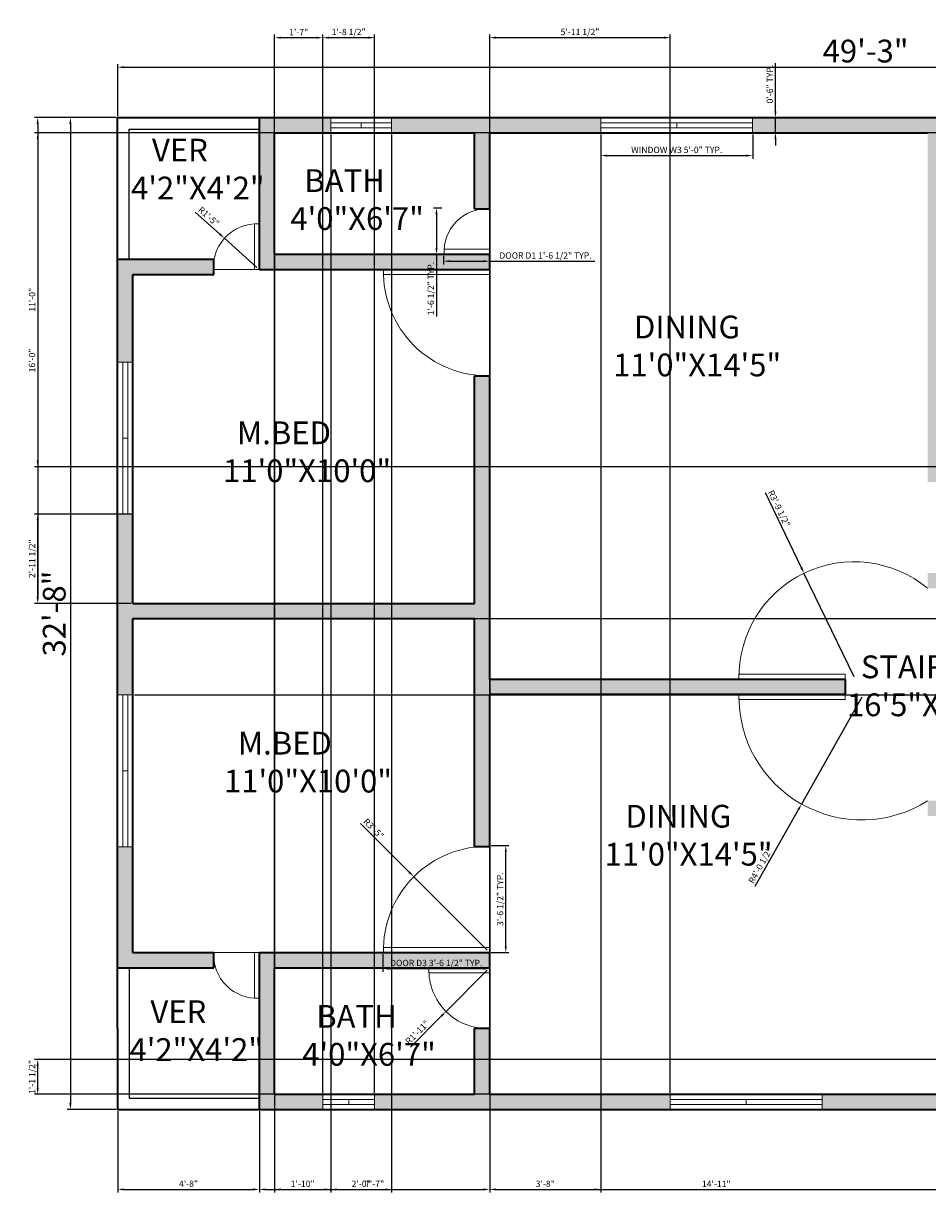
# Model space of a CAD drawing. Units: inches. Extents: x 5145 to 5807, y 9597 to 10060.
# Tile 1 of 3: x 5145 to 5502, y 9597 to 10060. Entities that reach past the tile are written whole.
import ezdxf

# ---------------------------------------------------------------- set-up
doc = ezdxf.new("R2010")
doc.units = ezdxf.units.IN
for name, color, linetype, lineweight in [('A-ANNO-DIMS', 7, 'Continuous', 18), ('A-AREA-IDEN', 7, 'Continuous', 18), ('A-GLAZ', 140, 'Continuous', 18), ('A-WALL', 7, 'Continuous', 35)]:
    doc.layers.add(name, color=color, linetype=linetype, lineweight=lineweight)
for name, color, linetype, lineweight, true_color in [('A-DOOR', 2, 'Continuous', 18, 0xf1eb1f), ('A-WALL-PATT', 159, 'Continuous', 13, 0x22346e), ('A-WALL-PRPT', 61, 'Continuous', 25, 0xedee99)]:
    doc.layers.add(name, color=color, linetype=linetype, lineweight=lineweight, true_color=true_color)
doc.styles.get("Standard").update_dxf_attribs({"font": 'arial.ttf'})
doc.dimstyles.new('ISO-25', dxfattribs={"dimtxt": 2.5, "dimasz": 2.5, "dimexe": 1.25, "dimexo": 0.625, "dimtad": 1, "dimlunit": 3, "dimtxsty": 'Standard', "dimcen": 2.5, "dimadec": 0, "dimazin": 0, "dimtfac": 1, "dimtmove": 0, "dimatfit": 3, "dimfxl": 1, "dimarcsym": 0})

# ---------------------------------------------------------------- blocks, each defined once
blk = doc.blocks.new('*D1')
at = {"layer": 'A-ANNO-DIMS', "color": 0, "lineweight": -2, "transparency": 16777216}
for p, q in [((5182.12, 10022.89), (5182.12, 10043.44)), ((5184.62, 10042.19), (5770.62, 10042.19)), ((5773.12, 10022.89), (5773.12, 10043.44))]:
    blk.add_line(p, q, dxfattribs=at)
at = {"layer": 'A-ANNO-DIMS', "color": 0, "transparency": 16777216}
for points in [[(5184.62, 10042.6), (5184.62, 10041.77), (5182.12, 10042.19)], [(5770.62, 10042.6), (5770.62, 10041.77), (5773.12, 10042.19)]]:
    blk.add_solid(points, dxfattribs=at)
at = {"layer": 'Defpoints', "color": 0, "transparency": 16777216}
for p in [(5773.12, 10042.19), (5182.12, 10022.27), (5773.12, 10022.27)]:
    blk.add_point(p, dxfattribs=at)
at = {"layer": 'A-ANNO-DIMS', "color": 0, "transparency": 16777216, "insert": (5477.62, 10047.41), "char_height": 9, "attachment_point": 5}
blk.add_mtext('49\'-3"', dxfattribs=at)
blk = doc.blocks.new('*D2')
at = {"layer": 'A-ANNO-DIMS', "color": 0, "lineweight": -2, "transparency": 16777216}
for p, q in [((5181.49, 10022.27), (5162.2, 10022.27)), ((5163.45, 10019.77), (5163.45, 9632.77)), ((5181.49, 9630.27), (5162.2, 9630.27))]:
    blk.add_line(p, q, dxfattribs=at)
at = {"layer": 'A-ANNO-DIMS', "color": 0, "transparency": 16777216}
for points in [[(5163.03, 10019.77), (5163.86, 10019.77), (5163.45, 10022.27)], [(5163.03, 9632.77), (5163.86, 9632.77), (5163.45, 9630.27)]]:
    blk.add_solid(points, dxfattribs=at)
at = {"layer": 'Defpoints', "color": 0, "transparency": 16777216}
for p in [(5182.12, 10022.27), (5163.45, 9630.27), (5182.12, 9630.27)]:
    blk.add_point(p, dxfattribs=at)
at = {"layer": 'A-ANNO-DIMS', "color": 0, "transparency": 16777216, "insert": (5158.22, 9826.27), "char_height": 9, "attachment_point": 5, "rotation": 90}
blk.add_mtext('32\'-8"', dxfattribs=at)
blk = doc.blocks.new('WIN-60IN')
for p, q in [((0, 6), (0, 0)), ((0, 6), (60, 6)), ((60, 0), (60, 6)), ((0, 4), (60, 4)), ((0, 2), (60, 2)), ((60, 0), (0, 0)), ((30, 2), (30, 4))]:
    blk.add_line(p, q)
blk = doc.blocks.new('DOOR-SWING-18IN')
for p, q in [((0.03, 18.03), (18.03, 18.03)), ((16.03, 0.03), (16.03, 18.03)), ((16.03, 18.03), (18.03, 18.03)), ((18.03, 18.03), (18.03, 0.03)), ((18.03, 0.03), (16.03, 0.03))]:
    blk.add_line(p, q)
blk.add_arc((17.03, 17.03), 17.03, 176.6335, 273.3665)
blk = doc.blocks.new('DOOR-SWING-42IN')
for p, q in [((42.01, 0), (42.01, 42)), ((0.01, 0), (0.01, 2)), ((0.01, 2), (42.01, 2)), ((42.01, 0), (0.01, 0)), ((42.01, 2), (42.01, 0))]:
    blk.add_line(p, q)
blk.add_arc((41.01, 1), 41.01, 88.6028, 181.3972)
blk = doc.blocks.new('*D13')
at = {"layer": 'A-ANNO-DIMS', "color": 0, "lineweight": -2, "transparency": 16777216}
for p, q in [((5373, 10015.64), (5373, 10006.02)), ((5433, 10015.64), (5433, 10006.02)), ((5375.5, 10007.27), (5430.5, 10007.27))]:
    blk.add_line(p, q, dxfattribs=at)
at = {"layer": 'A-ANNO-DIMS', "color": 0, "transparency": 16777216}
for points in [[(5375.5, 10007.68), (5375.5, 10006.85), (5373, 10007.27)], [(5430.5, 10007.68), (5430.5, 10006.85), (5433, 10007.27)]]:
    blk.add_solid(points, dxfattribs=at)
at = {"layer": 'Defpoints', "color": 0, "transparency": 16777216}
for p in [(5373, 10016.27), (5433, 10016.27), (5433, 10007.27)]:
    blk.add_point(p, dxfattribs=at)
at = {"layer": 'A-ANNO-DIMS', "color": 0, "transparency": 16777216, "insert": (5403, 10009.19), "char_height": 2.5, "attachment_point": 5}
blk.add_mtext('WINDOW W3 5\'-0" TYP.', dxfattribs=at)
blk = doc.blocks.new('*D14')
at = {"layer": 'A-ANNO-DIMS', "color": 0, "lineweight": -2, "transparency": 16777216}
for p, q in [((5442, 10024.77), (5442, 10043.76)), ((5433.62, 10022.27), (5443.25, 10022.27)), ((5442, 10016.27), (5442, 10022.27)), ((5433.62, 10016.27), (5443.25, 10016.27)), ((5442, 10013.77), (5442, 10011.27))]:
    blk.add_line(p, q, dxfattribs=at)
at = {"layer": 'A-ANNO-DIMS', "color": 0, "transparency": 16777216}
for points in [[(5441.58, 10024.77), (5442.41, 10024.77), (5442, 10022.27)], [(5441.58, 10013.77), (5442.41, 10013.77), (5442, 10016.27)]]:
    blk.add_solid(points, dxfattribs=at)
at = {"layer": 'Defpoints', "color": 0, "transparency": 16777216}
for p in [(5433, 10022.27), (5442, 10022.27), (5433, 10016.27)]:
    blk.add_point(p, dxfattribs=at)
at = {"layer": 'A-ANNO-DIMS', "color": 0, "transparency": 16777216, "insert": (5440.09, 10035.51), "char_height": 2.5, "attachment_point": 5, "rotation": 90}
blk.add_mtext('0\'-6" TYP.', dxfattribs=at)
blk = doc.blocks.new('*D15')
at = {"layer": 'A-ANNO-DIMS', "color": 0, "lineweight": -2, "transparency": 16777216}
for p, q in [((5310.83, 9967.64), (5310.83, 9964.27)), ((5329.12, 9967.64), (5329.12, 9964.27)), ((5313.33, 9965.52), (5326.62, 9965.52)), ((5329.12, 9965.52), (5370.69, 9965.52))]:
    blk.add_line(p, q, dxfattribs=at)
at = {"layer": 'A-ANNO-DIMS', "color": 0, "transparency": 16777216}
for points in [[(5313.33, 9965.94), (5313.33, 9965.11), (5310.83, 9965.52)], [(5326.62, 9965.94), (5326.62, 9965.11), (5329.12, 9965.52)]]:
    blk.add_solid(points, dxfattribs=at)
at = {"layer": 'Defpoints', "color": 0, "transparency": 16777216}
for p in [(5310.83, 9968.27), (5329.12, 9968.27), (5329.12, 9965.52)]:
    blk.add_point(p, dxfattribs=at)
at = {"layer": 'A-ANNO-DIMS', "color": 0, "transparency": 16777216, "insert": (5351.15, 9967.44), "char_height": 2.5, "attachment_point": 5}
blk.add_mtext('DOOR D1 1\'-6 1/2" TYP.', dxfattribs=at)
blk = doc.blocks.new('*D16')
at = {"layer": 'A-ANNO-DIMS', "color": 0, "lineweight": -2, "transparency": 16777216}
for p, q in [((5310.21, 9986.55), (5306.84, 9986.55)), ((5308.09, 9984.05), (5308.09, 9970.77)), ((5310.21, 9968.27), (5306.84, 9968.27)), ((5308.09, 9968.27), (5308.09, 9943.69))]:
    blk.add_line(p, q, dxfattribs=at)
at = {"layer": 'A-ANNO-DIMS', "color": 0, "transparency": 16777216}
for points in [[(5307.67, 9984.05), (5308.5, 9984.05), (5308.09, 9986.55)], [(5307.67, 9970.77), (5308.5, 9970.77), (5308.09, 9968.27)]]:
    blk.add_solid(points, dxfattribs=at)
at = {"layer": 'Defpoints', "color": 0, "transparency": 16777216}
for p in [(5310.83, 9986.55), (5308.09, 9968.27), (5310.83, 9968.27)]:
    blk.add_point(p, dxfattribs=at)
at = {"layer": 'A-ANNO-DIMS', "color": 0, "transparency": 16777216, "insert": (5306.17, 9954.73), "char_height": 2.5, "attachment_point": 5, "rotation": 90}
blk.add_mtext('1\'-6 1/2" TYP.', dxfattribs=at)
blk = doc.blocks.new('*D19')
at = {"layer": 'A-ANNO-DIMS', "color": 0, "lineweight": -2, "transparency": 16777216}
for p, q in [((5286.84, 9691.64), (5286.84, 9684.68)), ((5329.12, 9691.64), (5329.12, 9684.68)), ((5289.34, 9685.93), (5326.62, 9685.93))]:
    blk.add_line(p, q, dxfattribs=at)
at = {"layer": 'A-ANNO-DIMS', "color": 0, "transparency": 16777216}
for points in [[(5289.34, 9686.34), (5289.34, 9685.51), (5286.84, 9685.93)], [(5326.62, 9686.34), (5326.62, 9685.51), (5329.12, 9685.93)]]:
    blk.add_solid(points, dxfattribs=at)
at = {"layer": 'Defpoints', "color": 0, "transparency": 16777216}
for p in [(5286.84, 9692.27), (5329.12, 9692.27), (5329.12, 9685.93)]:
    blk.add_point(p, dxfattribs=at)
at = {"layer": 'A-ANNO-DIMS', "color": 0, "transparency": 16777216, "insert": (5307.98, 9687.85), "char_height": 2.5, "attachment_point": 5}
blk.add_mtext('DOOR D3 3\'-6 1/2" TYP.', dxfattribs=at)
blk = doc.blocks.new('*D20')
at = {"layer": 'A-ANNO-DIMS', "color": 0, "lineweight": -2, "transparency": 16777216}
for p, q in [((5329.74, 9734.54), (5336.71, 9734.54)), ((5335.46, 9694.77), (5335.46, 9732.04)), ((5329.74, 9692.27), (5336.71, 9692.27))]:
    blk.add_line(p, q, dxfattribs=at)
at = {"layer": 'A-ANNO-DIMS', "color": 0, "transparency": 16777216}
for points in [[(5335.04, 9732.04), (5335.87, 9732.04), (5335.46, 9734.54)], [(5335.04, 9694.77), (5335.87, 9694.77), (5335.46, 9692.27)]]:
    blk.add_solid(points, dxfattribs=at)
at = {"layer": 'Defpoints', "color": 0, "transparency": 16777216}
for p in [(5329.12, 9734.54), (5335.46, 9734.54), (5329.12, 9692.27)]:
    blk.add_point(p, dxfattribs=at)
at = {"layer": 'A-ANNO-DIMS', "color": 0, "transparency": 16777216, "insert": (5333.54, 9713.4), "char_height": 2.5, "attachment_point": 5, "rotation": 90}
blk.add_mtext('3\'-6 1/2" TYP.', dxfattribs=at)
blk = doc.blocks.new('*D21')
at = {"layer": 'A-ANNO-DIMS', "color": 0, "lineweight": -2, "transparency": 16777216}
for p, q in [((5182.12, 9629.64), (5182.12, 9597.42)), ((5238.12, 9629.64), (5238.12, 9597.42)), ((5184.62, 9598.67), (5235.62, 9598.67))]:
    blk.add_line(p, q, dxfattribs=at)
at = {"layer": 'A-ANNO-DIMS', "color": 0, "transparency": 16777216}
for points in [[(5184.62, 9599.08), (5184.62, 9598.25), (5182.12, 9598.67)], [(5235.62, 9599.08), (5235.62, 9598.25), (5238.12, 9598.67)]]:
    blk.add_solid(points, dxfattribs=at)
at = {"layer": 'Defpoints', "color": 0, "transparency": 16777216}
for p in [(5182.12, 9630.27), (5238.12, 9630.27), (5238.12, 9598.67)]:
    blk.add_point(p, dxfattribs=at)
at = {"layer": 'A-ANNO-DIMS', "color": 0, "transparency": 16777216, "insert": (5210.12, 9600.57), "char_height": 2.5, "attachment_point": 5}
blk.add_mtext('4\'-8"', dxfattribs=at)
blk = doc.blocks.new('*D22')
at = {"layer": 'A-ANNO-DIMS', "color": 0, "lineweight": -2, "transparency": 16777216}
for p, q in [((5329.12, 9635.64), (5329.12, 9597.42)), ((5238.12, 9629.64), (5238.12, 9597.42)), ((5240.62, 9598.67), (5326.62, 9598.67))]:
    blk.add_line(p, q, dxfattribs=at)
at = {"layer": 'A-ANNO-DIMS', "color": 0, "transparency": 16777216}
for points in [[(5240.62, 9599.08), (5240.62, 9598.25), (5238.12, 9598.67)], [(5326.62, 9599.08), (5326.62, 9598.25), (5329.12, 9598.67)]]:
    blk.add_solid(points, dxfattribs=at)
at = {"layer": 'Defpoints', "color": 0, "transparency": 16777216}
for p in [(5329.12, 9636.27), (5238.12, 9630.27), (5329.12, 9598.67)]:
    blk.add_point(p, dxfattribs=at)
at = {"layer": 'A-ANNO-DIMS', "color": 0, "transparency": 16777216, "insert": (5283.62, 9600.54), "char_height": 2.5, "attachment_point": 5}
blk.add_mtext('7\'-7"', dxfattribs=at)
blk = doc.blocks.new('*D23')
at = {"layer": 'A-ANNO-DIMS', "color": 0, "lineweight": -2, "transparency": 16777216}
for p, q in [((5329.12, 9635.64), (5329.12, 9597.42)), ((5508.12, 9635.64), (5508.12, 9597.42)), ((5331.62, 9598.67), (5505.62, 9598.67))]:
    blk.add_line(p, q, dxfattribs=at)
at = {"layer": 'A-ANNO-DIMS', "color": 0, "transparency": 16777216}
for points in [[(5331.62, 9599.08), (5331.62, 9598.25), (5329.12, 9598.67)], [(5505.62, 9599.08), (5505.62, 9598.25), (5508.12, 9598.67)]]:
    blk.add_solid(points, dxfattribs=at)
at = {"layer": 'Defpoints', "color": 0, "transparency": 16777216}
for p in [(5329.12, 9636.27), (5508.12, 9636.27), (5508.12, 9598.67)]:
    blk.add_point(p, dxfattribs=at)
at = {"layer": 'A-ANNO-DIMS', "color": 0, "transparency": 16777216, "insert": (5418.62, 9600.55), "char_height": 2.5, "attachment_point": 5}
blk.add_mtext('14\'-11"', dxfattribs=at)
blk = doc.blocks.new('*D29')
at = {"layer": 'A-ANNO-DIMS', "color": 0, "lineweight": -2, "transparency": 16777216}
for p, q in [((5590.49, 10016.27), (5149.27, 10016.27)), ((5150.52, 10013.77), (5150.52, 9886.77)), ((5590.49, 9884.27), (5149.27, 9884.27))]:
    blk.add_line(p, q, dxfattribs=at)
at = {"layer": 'A-ANNO-DIMS', "color": 0, "transparency": 16777216}
for points in [[(5150.1, 10013.77), (5150.93, 10013.77), (5150.52, 10016.27)], [(5150.1, 9886.77), (5150.93, 9886.77), (5150.52, 9884.27)]]:
    blk.add_solid(points, dxfattribs=at)
at = {"layer": 'Defpoints', "color": 0, "transparency": 16777216}
for p in [(5591.12, 10016.27), (5150.52, 9884.27), (5591.12, 9884.27)]:
    blk.add_point(p, dxfattribs=at)
at = {"layer": 'A-ANNO-DIMS', "color": 0, "transparency": 16777216, "insert": (5148.61, 9950.27), "char_height": 2.5, "attachment_point": 5, "rotation": 90}
blk.add_mtext('11\'-0"', dxfattribs=at)
blk = doc.blocks.new('*D33')
at = {"layer": 'A-ANNO-DIMS', "color": 0, "lineweight": -2, "transparency": 16777216}
for p, q in [((5181.49, 10022.27), (5149.27, 10022.27)), ((5150.52, 10019.77), (5150.52, 9832.77)), ((5187.49, 9830.27), (5149.27, 9830.27))]:
    blk.add_line(p, q, dxfattribs=at)
at = {"layer": 'A-ANNO-DIMS', "color": 0, "transparency": 16777216}
for points in [[(5150.1, 10019.77), (5150.93, 10019.77), (5150.52, 10022.27)], [(5150.1, 9832.77), (5150.93, 9832.77), (5150.52, 9830.27)]]:
    blk.add_solid(points, dxfattribs=at)
at = {"layer": 'Defpoints', "color": 0, "transparency": 16777216}
for p in [(5182.12, 10022.27), (5150.52, 9830.27), (5188.12, 9830.27)]:
    blk.add_point(p, dxfattribs=at)
at = {"layer": 'A-ANNO-DIMS', "color": 0, "transparency": 16777216, "insert": (5148.61, 9926.27), "char_height": 2.5, "attachment_point": 5, "rotation": 90}
blk.add_mtext('16\'-0"', dxfattribs=at)
blk = doc.blocks.new('*D34')
at = {"layer": 'A-ANNO-DIMS', "color": 0, "lineweight": -2, "transparency": 16777216}
for p, q in [((5244.12, 10015.64), (5244.12, 9597.42)), ((5266.31, 10015.64), (5266.31, 9597.42)), ((5246.62, 9598.67), (5263.81, 9598.67))]:
    blk.add_line(p, q, dxfattribs=at)
at = {"layer": 'A-ANNO-DIMS', "color": 0, "transparency": 16777216}
for points in [[(5246.62, 9599.08), (5246.62, 9598.25), (5244.12, 9598.67)], [(5263.81, 9599.08), (5263.81, 9598.25), (5266.31, 9598.67)]]:
    blk.add_solid(points, dxfattribs=at)
at = {"layer": 'Defpoints', "color": 0, "transparency": 16777216}
for p in [(5244.12, 10016.27), (5266.31, 10016.27), (5266.31, 9598.67)]:
    blk.add_point(p, dxfattribs=at)
at = {"layer": 'A-ANNO-DIMS', "color": 0, "transparency": 16777216, "insert": (5255.21, 9600.57), "char_height": 2.5, "attachment_point": 5}
blk.add_mtext('1\'-10"', dxfattribs=at)
blk = doc.blocks.new('*D35')
at = {"layer": 'A-ANNO-DIMS', "color": 0, "lineweight": -2, "transparency": 16777216}
for p, q in [((5266.31, 10015.64), (5266.31, 9597.42)), ((5290.31, 10015.64), (5290.31, 9597.42)), ((5268.81, 9598.67), (5287.81, 9598.67))]:
    blk.add_line(p, q, dxfattribs=at)
at = {"layer": 'A-ANNO-DIMS', "color": 0, "transparency": 16777216}
for points in [[(5268.81, 9599.08), (5268.81, 9598.25), (5266.31, 9598.67)], [(5287.81, 9599.08), (5287.81, 9598.25), (5290.31, 9598.67)]]:
    blk.add_solid(points, dxfattribs=at)
at = {"layer": 'Defpoints', "color": 0, "transparency": 16777216}
for p in [(5266.31, 10016.27), (5290.31, 10016.27), (5290.31, 9598.67)]:
    blk.add_point(p, dxfattribs=at)
at = {"layer": 'A-ANNO-DIMS', "color": 0, "transparency": 16777216, "insert": (5278.31, 9600.57), "char_height": 2.5, "attachment_point": 5}
blk.add_mtext('2\'-0"', dxfattribs=at)
blk = doc.blocks.new('*D36')
at = {"layer": 'A-ANNO-DIMS', "color": 0, "lineweight": -2, "transparency": 16777216}
for p, q in [((5329.12, 10015.64), (5329.12, 9597.42)), ((5373, 10015.64), (5373, 9597.42)), ((5331.62, 9598.67), (5370.5, 9598.67))]:
    blk.add_line(p, q, dxfattribs=at)
at = {"layer": 'A-ANNO-DIMS', "color": 0, "transparency": 16777216}
for points in [[(5331.62, 9599.08), (5331.62, 9598.25), (5329.12, 9598.67)], [(5370.5, 9599.08), (5370.5, 9598.25), (5373, 9598.67)]]:
    blk.add_solid(points, dxfattribs=at)
at = {"layer": 'Defpoints', "color": 0, "transparency": 16777216}
for p in [(5329.12, 10016.27), (5373, 10016.27), (5373, 9598.67)]:
    blk.add_point(p, dxfattribs=at)
at = {"layer": 'A-ANNO-DIMS', "color": 0, "transparency": 16777216, "insert": (5351.06, 9600.57), "char_height": 2.5, "attachment_point": 5}
blk.add_mtext('3\'-8"', dxfattribs=at)
blk = doc.blocks.new('*D40')
at = {"layer": 'A-ANNO-DIMS', "color": 0, "lineweight": -2, "transparency": 16777216}
for p, q in [((5244.12, 9636.89), (5244.12, 10055.12)), ((5246.62, 10053.87), (5260.67, 10053.87)), ((5263.17, 9636.89), (5263.17, 10055.12))]:
    blk.add_line(p, q, dxfattribs=at)
at = {"layer": 'A-ANNO-DIMS', "color": 0, "transparency": 16777216}
for points in [[(5246.62, 10054.28), (5246.62, 10053.45), (5244.12, 10053.87)], [(5260.67, 10054.28), (5260.67, 10053.45), (5263.17, 10053.87)]]:
    blk.add_solid(points, dxfattribs=at)
at = {"layer": 'Defpoints', "color": 0, "transparency": 16777216}
for p in [(5263.17, 10053.87), (5244.12, 9636.27), (5263.17, 9636.27)]:
    blk.add_point(p, dxfattribs=at)
at = {"layer": 'A-ANNO-DIMS', "color": 0, "transparency": 16777216, "insert": (5253.64, 10055.75), "char_height": 2.5, "attachment_point": 5}
blk.add_mtext('1\'-7"', dxfattribs=at)
blk = doc.blocks.new('*D41')
at = {"layer": 'A-ANNO-DIMS', "color": 0, "lineweight": -2, "transparency": 16777216}
for p, q in [((5263.17, 9636.89), (5263.17, 10055.12)), ((5265.67, 10053.87), (5281.12, 10053.87)), ((5283.62, 9636.89), (5283.62, 10055.12))]:
    blk.add_line(p, q, dxfattribs=at)
at = {"layer": 'A-ANNO-DIMS', "color": 0, "transparency": 16777216}
for points in [[(5265.67, 10054.28), (5265.67, 10053.45), (5263.17, 10053.87)], [(5281.12, 10054.28), (5281.12, 10053.45), (5283.62, 10053.87)]]:
    blk.add_solid(points, dxfattribs=at)
at = {"layer": 'Defpoints', "color": 0, "transparency": 16777216}
for p in [(5283.62, 10053.87), (5263.17, 9636.27), (5283.62, 9636.27)]:
    blk.add_point(p, dxfattribs=at)
at = {"layer": 'A-ANNO-DIMS', "color": 0, "transparency": 16777216, "insert": (5273.39, 10055.79), "char_height": 2.5, "attachment_point": 5}
blk.add_mtext('1\'-8 1/2"', dxfattribs=at)
blk = doc.blocks.new('*D42')
at = {"layer": 'A-ANNO-DIMS', "color": 0, "lineweight": -2, "transparency": 16777216}
for p, q in [((5329.12, 9636.89), (5329.12, 10055.12)), ((5331.62, 10053.87), (5397.94, 10053.87)), ((5400.44, 9636.89), (5400.44, 10055.12))]:
    blk.add_line(p, q, dxfattribs=at)
at = {"layer": 'A-ANNO-DIMS', "color": 0, "transparency": 16777216}
for points in [[(5331.62, 10054.28), (5331.62, 10053.45), (5329.12, 10053.87)], [(5397.94, 10054.28), (5397.94, 10053.45), (5400.44, 10053.87)]]:
    blk.add_solid(points, dxfattribs=at)
at = {"layer": 'Defpoints', "color": 0, "transparency": 16777216}
for p in [(5400.44, 10053.87), (5329.12, 9636.27), (5400.44, 9636.27)]:
    blk.add_point(p, dxfattribs=at)
at = {"layer": 'A-ANNO-DIMS', "color": 0, "transparency": 16777216, "insert": (5364.78, 10055.79), "char_height": 2.5, "attachment_point": 5}
blk.add_mtext('5\'-11 1/2"', dxfattribs=at)
blk = doc.blocks.new('*D45')
at = {"layer": 'A-ANNO-DIMS', "color": 0, "lineweight": -2, "transparency": 16777216}
for p, q in [((5187.49, 9865.61), (5149.27, 9865.61)), ((5150.52, 9832.77), (5150.52, 9863.11)), ((5187.49, 9830.27), (5149.27, 9830.27))]:
    blk.add_line(p, q, dxfattribs=at)
at = {"layer": 'A-ANNO-DIMS', "color": 0, "transparency": 16777216}
for points in [[(5150.1, 9863.11), (5150.93, 9863.11), (5150.52, 9865.61)], [(5150.1, 9832.77), (5150.93, 9832.77), (5150.52, 9830.27)]]:
    blk.add_solid(points, dxfattribs=at)
at = {"layer": 'Defpoints', "color": 0, "transparency": 16777216}
for p in [(5150.52, 9865.61), (5188.12, 9865.61), (5188.12, 9830.27)]:
    blk.add_point(p, dxfattribs=at)
at = {"layer": 'A-ANNO-DIMS', "color": 0, "transparency": 16777216, "insert": (5148.6, 9847.94), "char_height": 2.5, "attachment_point": 5, "rotation": 90}
blk.add_mtext('2\'-11 1/2"', dxfattribs=at)
blk = doc.blocks.new('*D46')
at = {"layer": 'A-ANNO-DIMS', "color": 0, "lineweight": -2, "transparency": 16777216}
for p, q in [((5188.74, 9824.27), (5805.97, 9824.27)), ((5804.72, 9821.77), (5804.72, 9796.64)), ((5188.74, 9794.14), (5805.97, 9794.14))]:
    blk.add_line(p, q, dxfattribs=at)
at = {"layer": 'A-ANNO-DIMS', "color": 0, "transparency": 16777216}
for points in [[(5804.3, 9821.77), (5805.13, 9821.77), (5804.72, 9824.27)], [(5804.3, 9796.64), (5805.13, 9796.64), (5804.72, 9794.14)]]:
    blk.add_solid(points, dxfattribs=at)
at = {"layer": 'Defpoints', "color": 0, "transparency": 16777216}
for p in [(5188.12, 9824.27), (5188.12, 9794.14), (5804.72, 9794.14)]:
    blk.add_point(p, dxfattribs=at)
at = {"layer": 'A-ANNO-DIMS', "color": 0, "transparency": 16777216, "insert": (5802.81, 9809.2), "char_height": 2.5, "attachment_point": 5, "rotation": 90}
blk.add_mtext('2\'-6"', dxfattribs=at)
blk = doc.blocks.new('*D49')
at = {"layer": 'A-ANNO-DIMS', "color": 0, "lineweight": -2, "transparency": 16777216}
for p, q in [((5724.49, 9649.99), (5149.27, 9649.99)), ((5150.52, 9638.77), (5150.52, 9647.49)), ((5724.49, 9636.27), (5149.27, 9636.27))]:
    blk.add_line(p, q, dxfattribs=at)
at = {"layer": 'A-ANNO-DIMS', "color": 0, "transparency": 16777216}
for points in [[(5150.1, 9647.49), (5150.93, 9647.49), (5150.52, 9649.99)], [(5150.1, 9638.77), (5150.93, 9638.77), (5150.52, 9636.27)]]:
    blk.add_solid(points, dxfattribs=at)
at = {"layer": 'Defpoints', "color": 0, "transparency": 16777216}
for p in [(5150.52, 9649.99), (5725.12, 9649.99), (5725.12, 9636.27)]:
    blk.add_point(p, dxfattribs=at)
at = {"layer": 'A-ANNO-DIMS', "color": 0, "transparency": 16777216, "insert": (5148.6, 9643.13), "char_height": 2.5, "attachment_point": 5, "rotation": 90}
blk.add_mtext('1\'-1 1/2"', dxfattribs=at)
blk = doc.blocks.new('*D50')
at = {"layer": 'A-ANNO-DIMS', "color": 0, "lineweight": -2, "transparency": 16777216}
for p, q in [((5476.13, 9793.27), (5452.29, 9750.98)), ((5434.04, 9718.58), (5451.06, 9748.8))]:
    blk.add_line(p, q, dxfattribs=at)
at = {"layer": 'A-ANNO-DIMS', "color": 0, "transparency": 16777216}
blk.add_solid([(5450.7, 9749), (5451.43, 9748.59), (5452.29, 9750.98)], dxfattribs=at)
at = {"layer": 'Defpoints', "color": 0, "transparency": 16777216}
for p in [(5476.13, 9793.27), (5452.29, 9750.98)]:
    blk.add_point(p, dxfattribs=at)
at = {"layer": 'A-ANNO-DIMS', "color": 0, "transparency": 16777216, "insert": (5436.32, 9726.55), "char_height": 2.5, "attachment_point": 5, "rotation": 60.5951}
blk.add_mtext('R4\'-0 1/2"', dxfattribs=at)
blk = doc.blocks.new('*D51')
at = {"layer": 'A-ANNO-DIMS', "color": 0, "lineweight": -2, "transparency": 16777216}
for p, q in [((5437.91, 9874.05), (5452.19, 9844.48)), ((5473.07, 9801.27), (5453.28, 9842.22))]:
    blk.add_line(p, q, dxfattribs=at)
at = {"layer": 'A-ANNO-DIMS', "color": 0, "transparency": 16777216}
blk.add_solid([(5452.57, 9844.66), (5451.82, 9844.29), (5453.28, 9842.22)], dxfattribs=at)
at = {"layer": 'Defpoints', "color": 0, "transparency": 16777216}
for p in [(5453.28, 9842.22), (5473.07, 9801.27)]:
    blk.add_point(p, dxfattribs=at)
at = {"layer": 'A-ANNO-DIMS', "color": 0, "transparency": 16777216, "insert": (5443.14, 9867.63), "char_height": 2.5, "attachment_point": 5, "rotation": 295.7836}
blk.add_mtext('R3\'-9 1/2"', dxfattribs=at)
blk = doc.blocks.new('*D52')
at = {"layer": 'A-ANNO-DIMS', "color": 0, "lineweight": -2, "transparency": 16777216}
for p, q in [((5278.08, 9743.3), (5297.35, 9724.03)), ((5328.12, 9693.27), (5299.12, 9722.27))]:
    blk.add_line(p, q, dxfattribs=at)
at = {"layer": 'A-ANNO-DIMS', "color": 0, "transparency": 16777216}
blk.add_solid([(5297.64, 9724.33), (5297.05, 9723.74), (5299.12, 9722.27)], dxfattribs=at)
at = {"layer": 'Defpoints', "color": 0, "transparency": 16777216}
for p in [(5299.12, 9722.27), (5328.12, 9693.27)]:
    blk.add_point(p, dxfattribs=at)
at = {"layer": 'A-ANNO-DIMS', "color": 0, "transparency": 16777216, "insert": (5283.06, 9741.01), "char_height": 2.5, "attachment_point": 5, "rotation": 315.0008}
blk.add_mtext('R3\'-5"', dxfattribs=at)
blk = doc.blocks.new('*D56')
at = {"layer": 'A-ANNO-DIMS', "color": 0, "lineweight": -2, "transparency": 16777216}
for p, q in [((5328.12, 9685.27), (5311.84, 9668.99)), ((5297.75, 9654.9), (5310.07, 9667.22))]:
    blk.add_line(p, q, dxfattribs=at)
at = {"layer": 'A-ANNO-DIMS', "color": 0, "transparency": 16777216}
blk.add_solid([(5309.78, 9667.52), (5310.36, 9666.93), (5311.84, 9668.99)], dxfattribs=at)
at = {"layer": 'Defpoints', "color": 0, "transparency": 16777216}
for p in [(5328.12, 9685.27), (5311.84, 9668.99)]:
    blk.add_point(p, dxfattribs=at)
at = {"layer": 'A-ANNO-DIMS', "color": 0, "transparency": 16777216, "insert": (5300.74, 9660.55), "char_height": 2.5, "attachment_point": 5, "rotation": 45}
blk.add_mtext('R1\'-11"', dxfattribs=at)
blk = doc.blocks.new('*D57')
at = {"layer": 'A-ANNO-DIMS', "color": 0, "lineweight": -2, "transparency": 16777216}
for p, q in [((5212.8, 9984.95), (5222.45, 9976.27)), ((5237.12, 9963.07), (5224.31, 9974.59))]:
    blk.add_line(p, q, dxfattribs=at)
at = {"layer": 'A-ANNO-DIMS', "color": 0, "transparency": 16777216}
blk.add_solid([(5222.73, 9976.58), (5222.17, 9975.96), (5224.31, 9974.59)], dxfattribs=at)
at = {"layer": 'Defpoints', "color": 0, "transparency": 16777216}
for p in [(5224.31, 9974.59), (5237.12, 9963.07)]:
    blk.add_point(p, dxfattribs=at)
at = {"layer": 'A-ANNO-DIMS', "color": 0, "transparency": 16777216, "insert": (5217.9, 9982.92), "char_height": 2.5, "attachment_point": 5, "rotation": 318.0132}
blk.add_mtext('R1\'-5"', dxfattribs=at)

msp = doc.modelspace()

# ---------------------------------------------------------------- hatches: boundary and pattern name
at = {"layer": 'A-WALL-PATT'}
h = msp.add_hatch(color=256, dxfattribs=at)
h.dxf.hatch_style = 1
h.paths.add_polyline_path([(5244.116, 10016.267), (5266.307, 10016.267), (5266.307, 10022.267), (5238.116, 10022.267), (5238.116, 10017.767), (5238.116, 9962.267), (5329.116, 9962.267), (5329.116, 9968.267), (5311.116, 9968.267), (5244.116, 9968.267)])
h.paths.add_polyline_path([(5372.995, 10022.267), (5290.307, 10022.267), (5290.307, 10016.267), (5323.116, 10016.267), (5323.116, 9986.267), (5327.116, 9986.267, -0.0293864), (5329.116, 9986.267), (5329.116, 10016.267), (5372.995, 10016.267)])
h.paths.add_polyline_path([(5523.196, 10022.267), (5432.995, 10022.267), (5432.995, 10016.267), (5502.116, 10016.267), (5502.116, 9878.267), (5508.116, 9878.267), (5508.116, 9908.267), (5508.116, 10016.267), (5523.196, 10016.267)])
h.paths.add_polyline_path([(5623.247, 10022.267), (5559.196, 10022.267), (5559.196, 10016.267), (5591.116, 10016.267), (5591.116, 9884.267), (5538.116, 9884.267), (5538.116, 9880.267, -0.0172363), (5538.116, 9878.267), (5597.116, 9878.267), (5597.116, 10016.267), (5623.247, 10016.267)])
h.paths.add_polyline_path([(5731.116, 10022.267), (5695.247, 10022.267), (5695.247, 10016.267), (5725.116, 10016.267), (5725.116, 9968.267), (5731.116, 9968.267)])
h.paths.add_polyline_path([(5731.116, 9920.267), (5725.116, 9920.267), (5725.116, 9860.267, -0.0293864), (5727.116, 9860.267), (5731.116, 9860.267)])
h.paths.add_polyline_path([(5731.116, 9842.267), (5725.116, 9842.267), (5502.116, 9842.267), (5502.116, 9836.267), (5725.116, 9836.267), (5725.116, 9814.459), (5731.116, 9814.459)])
h.paths.add_polyline_path([(5731.116, 9778.459), (5725.116, 9778.459), (5725.116, 9752.267), (5502.116, 9752.267), (5502.116, 9746.267), (5731.116, 9746.267)])
h.paths.add_polyline_path([(5514.116, 9717.93), (5508.116, 9717.93), (5508.116, 9704.267), (5508.116, 9636.267), (5460.439, 9636.267), (5460.439, 9630.267), (5539.543, 9630.267), (5539.543, 9636.267), (5514.116, 9636.267), (5514.116, 9704.267)])
h.paths.add_polyline_path([(5603.116, 9717.93), (5544.116, 9717.93, -0.0172363), (5544.116, 9715.93), (5544.116, 9711.93), (5597.116, 9711.93), (5597.116, 9636.267), (5575.543, 9636.267), (5575.543, 9630.267), (5646.695, 9630.267), (5646.695, 9636.267), (5603.116, 9636.267), (5603.116, 9704.267)])
h.paths.add_polyline_path([(5731.116, 9649.987), (5725.116, 9649.987), (5725.116, 9636.267), (5694.695, 9636.267), (5694.695, 9630.267), (5731.116, 9630.267)])
h.paths.add_polyline_path([(5731.116, 9728.267), (5725.116, 9728.267), (5725.116, 9685.987), (5731.116, 9685.987)])
h.paths.add_polyline_path([(5400.439, 9636.267), (5329.116, 9636.267), (5329.116, 9662.267, -0.0217289), (5327.116, 9662.267), (5323.116, 9662.267), (5323.116, 9636.267), (5283.616, 9636.267), (5283.616, 9630.267), (5329.116, 9630.267), (5400.439, 9630.267)])
h.paths.add_polyline_path([(5263.165, 9636.267), (5244.116, 9636.267), (5244.116, 9686.267), (5329.116, 9686.267), (5329.116, 9692.267), (5287.116, 9692.267), (5238.116, 9692.267), (5238.116, 9674.267), (5238.116, 9630.267), (5263.165, 9630.267)])
h.paths.add_polyline_path([(5220.116, 9690.267, -0.0293864), (5220.116, 9692.267), (5188.116, 9692.267), (5188.116, 9734.135), (5182.116, 9734.135), (5182.116, 9686.267), (5220.116, 9686.267)])
h.paths.add_polyline_path([(5329.116, 9794.267), (5469.593, 9794.267), (5469.593, 9800.267), (5427.593, 9800.267), (5329.116, 9800.267), (5329.116, 9830.267), (5329.116, 9920.267, -0.0121933), (5327.116, 9920.267), (5323.116, 9920.267), (5323.116, 9830.267), (5188.116, 9830.267), (5188.116, 9865.614), (5182.116, 9865.614), (5182.116, 9794.135), (5188.116, 9794.135), (5188.116, 9824.267), (5323.116, 9824.267), (5323.116, 9734.267), (5327.116, 9734.267, -0.0121933), (5329.116, 9734.267)])
h = msp.add_hatch(color=256, dxfattribs=at)
h.dxf.hatch_style = 1
h.paths.add_polyline_path([(5188.116, 9960.267), (5220.116, 9960.267, -0.0818019), (5220.116, 9965.867), (5220.116, 9966.267), (5182.116, 9966.267), (5182.116, 9925.614), (5188.116, 9925.614)])

# ---------------------------------------------------------------- linework, layer by layer
at = {"layer": 'A-DOOR'}
for p, q in [((5238.116, 9980.267), (5236.116, 9980.267)), ((5236.116, 9980.267), (5236.116, 9962.267)), ((5238.116, 9962.267), (5238.116, 9980.267)), ((5220.116, 9962.267), (5238.116, 9962.267)), ((5236.116, 9962.267), (5238.116, 9962.267)), ((5427.593, 9800.267), (5427.593, 9802.267)), ((5427.593, 9802.267), (5469.593, 9802.267)), ((5469.593, 9802.267), (5469.593, 9800.267)), ((5469.593, 9800.267), (5427.593, 9800.267)), ((5469.593, 9794.267), (5427.593, 9794.267)), ((5427.593, 9794.267), (5427.593, 9792.267)), ((5427.593, 9792.267), (5469.593, 9792.267)), ((5469.593, 9792.267), (5469.593, 9794.267)), ((5329.116, 9686.267), (5305.116, 9686.267)), ((5305.116, 9686.267), (5305.116, 9684.267)), ((5329.116, 9684.267), (5329.116, 9686.267)), ((5329.116, 9686.267), (5329.116, 9662.267)), ((5305.116, 9684.267), (5329.116, 9684.267))]:
    msp.add_line(p, q, dxfattribs=at)
for centre, radius, start, end in [((5237.116, 9963.067), 17.229, 86.6726, 189.35298), ((5473.067, 9801.267), 45.485, 50.30762, 181.25976), ((5476.126, 9793.267), 48.544, 178.81962, 302.37097), ((5328.116, 9685.267), 23.022, 177.51045, 272.48955)]:
    msp.add_arc(centre, radius, start, end, dxfattribs=at)
at = {"layer": 'A-GLAZ'}
for p, q in [((5266.307, 10022.267), (5266.307, 10016.267)), ((5290.307, 10022.267), (5266.307, 10022.267)), ((5266.307, 10022.267), (5290.307, 10022.267)), ((5266.307, 10022.267), (5266.307, 10016.267)), ((5290.307, 10020.267), (5266.307, 10020.267)), ((5290.307, 10018.267), (5266.307, 10018.267)), ((5278.307, 10018.267), (5278.307, 10020.267)), ((5290.307, 10016.267), (5290.307, 10022.267)), ((5290.307, 10022.267), (5290.307, 10022.267)), ((5290.307, 10016.267), (5290.307, 10022.267)), ((5372.995, 10016.267), (5372.995, 10022.267)), ((5372.995, 10022.267), (5432.995, 10022.267)), ((5432.995, 10022.267), (5432.995, 10016.267)), ((5266.307, 10016.267), (5290.307, 10016.267)), ((5266.307, 10016.267), (5290.307, 10016.267)), ((5372.995, 10016.267), (5432.995, 10016.267)), ((5182.116, 9865.614), (5188.116, 9865.614)), ((5182.116, 9794.135), (5188.116, 9794.135)), ((5182.116, 9794.135), (5182.116, 9746.135)), ((5188.116, 9794.135), (5182.116, 9794.135)), ((5184.116, 9794.135), (5184.116, 9734.135)), ((5186.116, 9794.135), (5186.116, 9734.135)), ((5188.116, 9734.135), (5188.116, 9794.135)), ((5188.116, 9734.135), (5188.116, 9794.135)), ((5186.116, 9764.135), (5184.116, 9764.135)), ((5182.116, 9746.135), (5182.116, 9734.135)), ((5182.116, 9734.135), (5188.116, 9734.135)), ((5182.116, 9734.135), (5188.116, 9734.135)), ((5263.165, 9636.267), (5263.165, 9630.267)), ((5281.165, 9636.267), (5263.165, 9636.267)), ((5263.165, 9636.267), (5263.165, 9630.267)), ((5281.165, 9636.267), (5283.616, 9636.267)), ((5283.616, 9636.267), (5283.616, 9630.267)), ((5283.616, 9630.267), (5283.616, 9636.267)), ((5400.439, 9630.267), (5400.439, 9636.267)), ((5460.439, 9636.267), (5460.439, 9630.267)), ((5283.616, 9634.267), (5263.165, 9634.267)), ((5283.616, 9632.267), (5263.165, 9632.267)), ((5263.165, 9632.267), (5273.391, 9632.267)), ((5263.165, 9630.267), (5281.165, 9630.267)), ((5263.165, 9630.267), (5283.616, 9630.267)), ((5273.391, 9632.267), (5273.391, 9634.267)), ((5283.616, 9630.267), (5281.165, 9630.267)), ((5400.439, 9630.267), (5460.439, 9630.267))]:
    msp.add_line(p, q, dxfattribs=at)
at = {"layer": 'A-WALL'}
for p, q in [((5182.116, 10022.267), (5662.116, 10022.267)), ((5182.116, 9662.267), (5182.116, 10022.267)), ((5238.116, 9962.267), (5238.116, 10022.267)), ((5244.116, 10016.267), (5323.116, 10016.267)), ((5244.116, 9968.267), (5244.116, 10016.267)), ((5323.116, 9986.267), (5323.116, 10016.267)), ((5329.116, 9986.267), (5329.116, 10016.267)), ((5329.116, 10016.267), (5502.116, 10016.267)), ((5323.116, 9986.267), (5329.116, 9986.267)), ((5244.116, 9968.267), (5329.116, 9968.267)), ((5329.116, 9962.267), (5329.116, 9968.267)), ((5182.116, 9966.267), (5220.116, 9966.267)), ((5220.116, 9960.267), (5220.116, 9966.267)), ((5188.116, 9960.267), (5220.116, 9960.267)), ((5188.116, 9830.267), (5188.116, 9960.267)), ((5238.116, 9962.267), (5329.116, 9962.267)), ((5323.116, 9920.267), (5329.116, 9920.267)), ((5323.116, 9830.267), (5323.116, 9920.267)), ((5329.116, 9830.267), (5329.116, 9920.267)), ((5188.116, 9830.267), (5323.116, 9830.267)), ((5329.116, 9800.267), (5329.116, 9830.267)), ((5188.116, 9824.267), (5323.116, 9824.267)), ((5188.116, 9692.267), (5188.116, 9824.267)), ((5323.116, 9734.267), (5323.116, 9824.267)), ((5469.593, 9800.267), (5329.116, 9800.267)), ((5469.593, 9800.267), (5469.593, 9794.267)), ((5329.116, 9734.267), (5329.116, 9794.267)), ((5469.593, 9794.267), (5329.116, 9794.267)), ((5323.116, 9734.267), (5329.116, 9734.267)), ((5188.116, 9692.267), (5220.116, 9692.267)), ((5220.116, 9686.267), (5220.116, 9692.267)), ((5238.116, 9630.267), (5238.116, 9692.267)), ((5238.116, 9692.267), (5329.116, 9692.267)), ((5329.116, 9686.267), (5329.116, 9692.267)), ((5182.116, 9686.267), (5220.116, 9686.267)), ((5244.116, 9636.267), (5244.116, 9686.267)), ((5244.116, 9686.267), (5329.116, 9686.267)), ((5182.116, 9662.267), (5182.116, 9630.267)), ((5323.116, 9636.267), (5323.116, 9662.267)), ((5329.116, 9662.267), (5323.116, 9662.267)), ((5329.116, 9636.267), (5329.116, 9662.267)), ((5244.116, 9636.267), (5323.116, 9636.267)), ((5329.116, 9636.267), (5508.116, 9636.267)), ((5182.116, 9630.267), (5329.116, 9630.267)), ((5329.116, 9630.267), (5773.116, 9630.267))]:
    msp.add_line(p, q, dxfattribs=at)
at = {"layer": 'A-WALL-PRPT'}
for p, q in [((5238.116, 10022.267), (5182.116, 10022.267)), ((5182.116, 10022.267), (5182.116, 9966.267)), ((5238.116, 10017.767), (5238.116, 10022.267)), ((5186.616, 10017.767), (5238.116, 10017.767)), ((5186.616, 9966.267), (5186.616, 10017.767)), ((5186.616, 9966.267), (5186.616, 10017.767)), ((5186.616, 10017.767), (5238.116, 10017.767)), ((5182.116, 9686.267), (5182.116, 9630.267)), ((5186.616, 9686.267), (5186.616, 9634.767)), ((5186.616, 9686.267), (5186.616, 9634.767)), ((5186.616, 9634.767), (5238.116, 9634.767)), ((5186.616, 9634.767), (5238.116, 9634.767)), ((5182.116, 9630.267), (5238.116, 9630.267))]:
    msp.add_line(p, q, dxfattribs=at)

# ---------------------------------------------------------------- block references
at = {"layer": 'A-DOOR', "rotation": 270.0000000000104}
msp.add_blockref('DOOR-SWING-18IN', (5311.087, 9986.297), dxfattribs=at)
at = {"layer": 'A-DOOR', "extrusion": (0, 0, -1), "zscale": -1, "rotation": 180}
msp.add_blockref('DOOR-SWING-42IN', (-5287.104, 9962.268), dxfattribs=at)
at = {"layer": 'A-DOOR'}
for name, p in [('DOOR-SWING-42IN', (5287.104, 9692.267)), ('DOOR-SWING-18IN', (5220.087, 9674.238))]:
    msp.add_blockref(name, p, dxfattribs=at)
at = {"layer": 'A-GLAZ'}
msp.add_blockref('WIN-60IN', (5372.995, 10016.267), dxfattribs=at)
for p, rotation in [((5182.116, 9925.614), 269.9999999999966), ((5460.439, 9636.268), 180)]:
    msp.add_blockref('WIN-60IN', p, dxfattribs=dict(at, rotation=rotation))

# ---------------------------------------------------------------- texts
at = {"layer": 'A-AREA-IDEN', "char_height": 9, "attachment_point": 1}
for s, width, heights, insert in [('    VER\\P 4\'2"X4\'2"', 64.82808, [42.408], (5184.67, 10013.933)), ('   BATH\\P 4\'0"X6\'7"', 64.22217, [40.666], (5247.593, 10001.881)), ('    DINING\\P 11\'0"X14\'5"', 77.59661, [102.589], (5375.115, 9944.023)), ('  M.BED\\P11\'0"X10\'0"', 51.95741, [0], (5223.76, 9902.205)), ('  STAIR\\P16\'5"X7\'0"', 91.95952, [57.275], (5470.253, 9809.7)), ('  M.BED\\P11\'0"X10\'0"', 51.95741, [0], (5224.119, 9779.555)), ('    DINING\\P 11\'0"X14\'5"', 77.59661, [102.589], (5371.72, 9750.671)), ('    VER\\P 4\'2"X4\'2"', 64.82808, [42.408], (5184.047, 9673.446)), ('  BATH\\P4\'0"X6\'7"', 51.95741, [0], (5255.051, 9671.568))]:
    msp.add_mtext_dynamic_manual_height_columns(s, width=width, gutter_width=12.5, heights=heights, dxfattribs=dict(at, insert=insert))

# ---------------------------------------------------------------- dimensions: what is measured, and where the dimension line sits
at = {"layer": 'A-ANNO-DIMS'}
for base, p1, p2, picture, middle in [((5263.165, 10053.867), (5244.116, 9636.267), (5263.165, 9636.267), '*D40', (5253.641, 10055.748)), ((5283.616, 10053.867), (5263.165, 9636.267), (5283.616, 9636.267), '*D41', (5273.391, 10055.785)), ((5400.439, 10053.867), (5329.116, 9636.267), (5400.439, 9636.267), '*D42', (5364.778, 10055.785)), ((5266.307, 9598.667), (5244.116, 10016.267), (5266.307, 10016.267), '*D34', (5255.212, 9600.569)), ((5290.307, 9598.667), (5266.307, 10016.267), (5290.307, 10016.267), '*D35', (5278.307, 9600.569)), ((5372.995, 9598.667), (5329.116, 10016.267), (5372.995, 10016.267), '*D36', (5351.056, 9600.57)), ((5329.116, 9598.667), (5238.116, 9630.267), (5329.116, 9636.267), '*D22', (5283.616, 9600.542)), ((5508.116, 9598.667), (5329.116, 9636.267), (5508.116, 9636.267), '*D23', (5418.616, 9600.548)), ((5238.116, 9598.667), (5182.116, 9630.267), (5238.116, 9630.267), '*D21', (5210.116, 9600.569))]:
    dim = msp.add_linear_dim(base=base, p1=p1, p2=p2, dimstyle='ISO-25', override={"dimdec": 1, "dimlfac": 1, "dimrnd": 0, "dimzin": 1, "dimdsep": 46, "dimlunit": 4, "dimfrac": 2}, dxfattribs=at)
    dim.commit()
    dim.dimension.update_dxf_attribs({"geometry": picture, "text_midpoint": middle})
dim = msp.add_linear_dim(base=(5773.116, 10042.186), p1=(5182.116, 10022.267), p2=(5773.116, 10022.267), dimstyle='ISO-25', override={"dimtxt": 9, "dimclrd": 0, "dimclre": 0, "dimclrt": 0}, dxfattribs=at)
dim.commit()
dim.dimension.update_dxf_attribs({"geometry": '*D1', "text_midpoint": (5477.616, 10042.186), "dimtype": 160})
for base, p1, p2, angle, text, picture, middle in [((5441.995, 10022.267), (5432.995, 10016.267), (5432.995, 10022.267), 90, '<> TYP.', '*D14', (5440.094, 10035.512)), ((5308.088, 9968.267), (5310.831, 9986.553), (5310.831, 9968.267), 270, '<> TYP.', '*D16', (5306.17, 9954.728)), ((5329.116, 9965.525), (5310.831, 9968.267), (5329.116, 9968.267), 0, 'DOOR D1 <> TYP.', '*D15', (5351.153, 9967.443)), ((5335.457, 9734.541), (5329.116, 9692.267), (5329.116, 9734.541), 90, '<> TYP.', '*D20', (5333.539, 9713.404))]:
    dim = msp.add_linear_dim(base=base, p1=p1, p2=p2, angle=angle, text=text, dimstyle='ISO-25', override={"dimdec": 1, "dimlfac": 1, "dimrnd": 0, "dimzin": 1, "dimdsep": 46, "dimlunit": 4, "dimfrac": 2}, dxfattribs=at)
    dim.commit()
    dim.dimension.update_dxf_attribs({"geometry": picture, "text_midpoint": middle})
for base, p1, p2, override, picture, middle in [((5150.516, 9830.267), (5182.116, 10022.267), (5188.116, 9830.267), {"dimdec": 1, "dimlfac": 1, "dimrnd": 0, "dimzin": 1, "dimdsep": 46, "dimlunit": 4, "dimfrac": 2}, '*D33', (5148.615, 9926.267)), ((5163.445, 9630.267), (5182.116, 10022.267), (5182.116, 9630.267), {"dimtxt": 9, "dimclrd": 0, "dimclre": 0, "dimclrt": 0}, '*D2', (5158.222, 9826.267)), ((5150.516, 9884.267), (5591.116, 10016.267), (5591.116, 9884.267), {"dimdec": 1, "dimlfac": 1, "dimrnd": 0, "dimzin": 1, "dimdsep": 46, "dimlunit": 4, "dimfrac": 2}, '*D29', (5148.615, 9950.267)), ((5150.516, 9865.614), (5188.116, 9830.267), (5188.116, 9865.614), {"dimdec": 1, "dimlfac": 1, "dimrnd": 0, "dimzin": 1, "dimdsep": 46, "dimlunit": 4, "dimfrac": 2}, '*D45', (5148.599, 9847.941)), ((5804.716, 9794.135), (5188.116, 9824.267), (5188.116, 9794.135), {"dimdec": 1, "dimlfac": 1, "dimrnd": 0, "dimzin": 1, "dimdsep": 46, "dimlunit": 4, "dimfrac": 2}, '*D46', (5802.815, 9809.201)), ((5150.516, 9649.987), (5725.116, 9636.267), (5725.116, 9649.987), {"dimdec": 1, "dimlfac": 1, "dimrnd": 0, "dimzin": 1, "dimdsep": 46, "dimlunit": 4, "dimfrac": 2}, '*D49', (5148.599, 9643.127))]:
    dim = msp.add_linear_dim(base=base, p1=p1, p2=p2, angle=90, dimstyle='ISO-25', override=override, dxfattribs=at)
    dim.commit()
    dim.dimension.update_dxf_attribs({"geometry": picture, "text_midpoint": middle})
for base, p1, p2, text, picture, middle in [((5432.995, 10007.267), (5372.995, 10016.267), (5432.995, 10016.267), 'WINDOW W3 <> TYP.', '*D13', (5402.995, 10009.187)), ((5329.116, 9685.926), (5286.843, 9692.267), (5329.116, 9692.267), 'DOOR D3 <> TYP.', '*D19', (5307.98, 9687.846))]:
    dim = msp.add_linear_dim(base=base, p1=p1, p2=p2, text=text, dimstyle='ISO-25', override={"dimdec": 1, "dimlfac": 1, "dimrnd": 0, "dimzin": 1, "dimdsep": 46, "dimlunit": 4, "dimfrac": 2}, dxfattribs=at)
    dim.commit()
    dim.dimension.update_dxf_attribs({"geometry": picture, "text_midpoint": middle})
for center, mpoint, picture, middle in [((5237.116, 9963.067), (5224.31, 9974.593), '*D57', (5216.626, 9981.508)), ((5473.067, 9801.267), (5453.282, 9842.224), '*D51', (5441.411, 9866.798)), ((5476.126, 9793.267), (5452.292, 9750.977), '*D50', (5437.992, 9725.603)), ((5328.116, 9693.267), (5299.116, 9722.267), '*D52', (5281.716, 9739.667)), ((5328.116, 9685.267), (5311.838, 9668.989), '*D56', (5302.07, 9659.221))]:
    dim = msp.add_radius_dim(center=center, mpoint=mpoint, dimstyle='ISO-25', override={"dimdec": 1, "dimlfac": 1, "dimrnd": 0, "dimzin": 1, "dimdsep": 46, "dimlunit": 4, "dimfrac": 2}, dxfattribs=at)
    dim.commit()
    dim.dimension.update_dxf_attribs({"geometry": picture, "text_midpoint": middle, "dimtype": 164})

doc.saveas('drawing.dxf')
